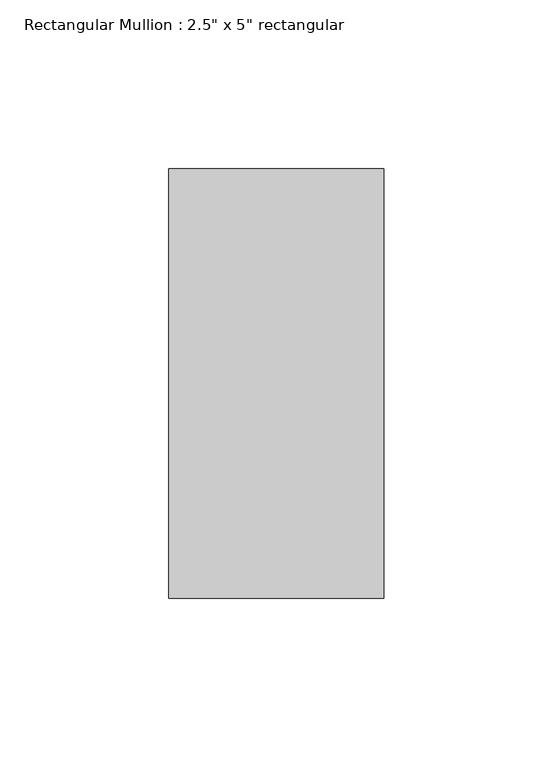
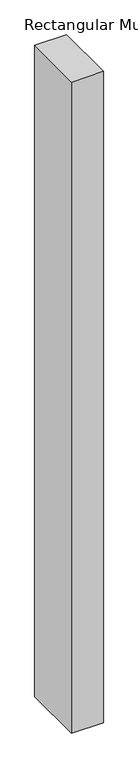
"""IFC4 building model written with IfcOpenShell, lengths in millimetres: member geometry."""

from ifc_helpers import new_model, si_unit, frame, origin, place, context, project, spatial, polyline, outline, extrude, source, transform, mapped, element, save


def member_c6627131(model_context):
    return source(origin(), model_context, "Body", "SweptSolid", [
        extrude(outline(polyline([(0.0, 63.5), (0.0, -63.5), (-63.5, -63.5), (-63.5, 63.5), (0.0, 63.5)])), frame((0.0, 0.0, -1371.6), z_axis=(0.0, 0.0, 1.0), x_axis=(1.0, 0.0, 0.0)), (0.0, 0.0, 1.0), 1371.6),
    ])


if __name__ == "__main__":
    model = new_model("IFC4")
    model_context = context("Model", 3, world=origin())
    ifc_project = project(units=[si_unit("LENGTHUNIT", "METRE", prefix="MILLI")], contexts=[model_context])
    site = spatial("IfcSite", under=ifc_project)
    building = spatial("IfcBuilding", under=site)
    placement = place(None, origin())
    member_shape = member_c6627131(model_context)
    element("IfcMember", 1, ObjectType="Rectangular Mullion : 2.5\" x 5\" rectangular", at=placement, inside=building, context=model_context, shape_type="MappedRepresentation", body=[
        mapped(member_shape, transform((0.0, 0.0, 0.0), x_axis=(1.0, 0.0, 0.0), y_axis=(0.0, 1.0, 0.0), z_axis=(0.0, 0.0, 1.0))),
    ])
    save(model, "model.ifc")

# Revit data of these elements
# Type "Rectangular Mullion : 2.5\" x 5\" rectangular"
#   built-in parameter 1007304 = 0.416667 (stored number, unit not read)
#   built-in parameter 1007301 = 0.104167 (stored number, unit not read)
#   built-in parameter 1007300 = 0.104167 (stored number, unit not read)
